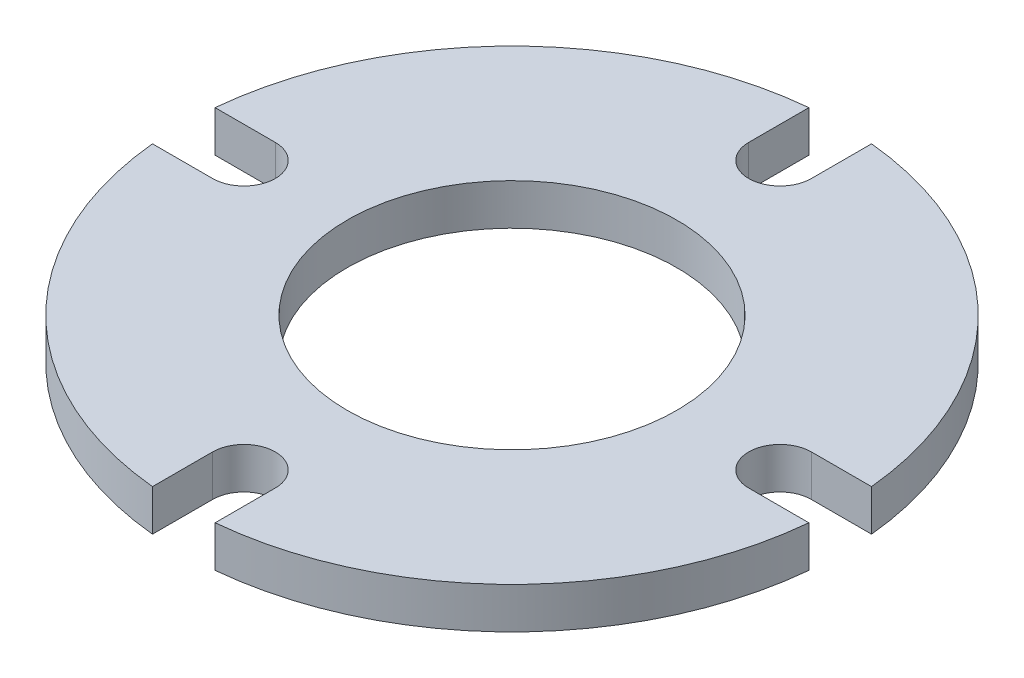
SolidWorks part; units mm, degrees
material "Plain Carbon Steel"
ref_plane "Front Plane" through (0, 0, 0) normal (0, 0, 1) x (1, 0, 0)
ref_plane "Top Plane" through (0, 0, 0) normal (0, 1, 0) x (1, 0, 0)
ref_plane "Right Plane" through (0, 0, 0) normal (1, 0, 0) x (0, 0, -1)
sketch "Disk Profile Sketch" plane through (0, 0, 0) normal (0, 1, 0) x (1, 0, 0)
  line L0 (0, -119.8312) -> (0, 143.762) construction
  line L1 (-103.0213, 0) -> (112.233, 0) construction
  line L2 (-9.5, 81.3) -> (-9.5, 99.5477)
  line L3 (9.5, 81.3) -> (9.5, 99.5477)
  line L4 (81.3, -9.5) -> (99.5477, -9.5)
  line L5 (81.3, 9.5) -> (99.5477, 9.5)
  line L6 (-9.5, -81.3) -> (-9.5, -99.5477)
  line L7 (9.5, -81.3) -> (9.5, -99.5477)
  line L8 (-81.3, 9.5) -> (-99.5477, 9.5)
  line L9 (-81.3, -9.5) -> (-99.5477, -9.5)
  circle A0 centre (0, 0) radius 50
  arc A1 (-9.5, 99.5477) -> (-99.5477, 9.5) centre (0, 0) ccw
  circle A2 centre (0, 0) radius 81.3 construction
  arc A3 (-9.5, 81.3) -> (9.5, 81.3) centre (0, 81.3) ccw
  arc A4 (81.3, 9.5) -> (81.3, -9.5) centre (81.3, 0) ccw
  arc A5 (9.5, -81.3) -> (-9.5, -81.3) centre (0, -81.3) ccw
  arc A6 (-81.3, -9.5) -> (-81.3, 9.5) centre (-81.3, 0) ccw
  arc A7 (-99.5477, -9.5) -> (-9.5, -99.5477) centre (0, 0) ccw
  arc A8 (9.5, -99.5477) -> (99.5477, -9.5) centre (0, 0) ccw
  arc A9 (99.5477, 9.5) -> (9.5, 99.5477) centre (0, 0) ccw
  dimension "D1" = 100
  dimension "D2" = 200
  dimension "D3" = 162.6
  dimension "D4" = 19
  dimension "D5" = 4
extrude "Slotted Disk Ø200x12.5" add sketch "Disk Profile Sketch" along normal mid plane 12.5
